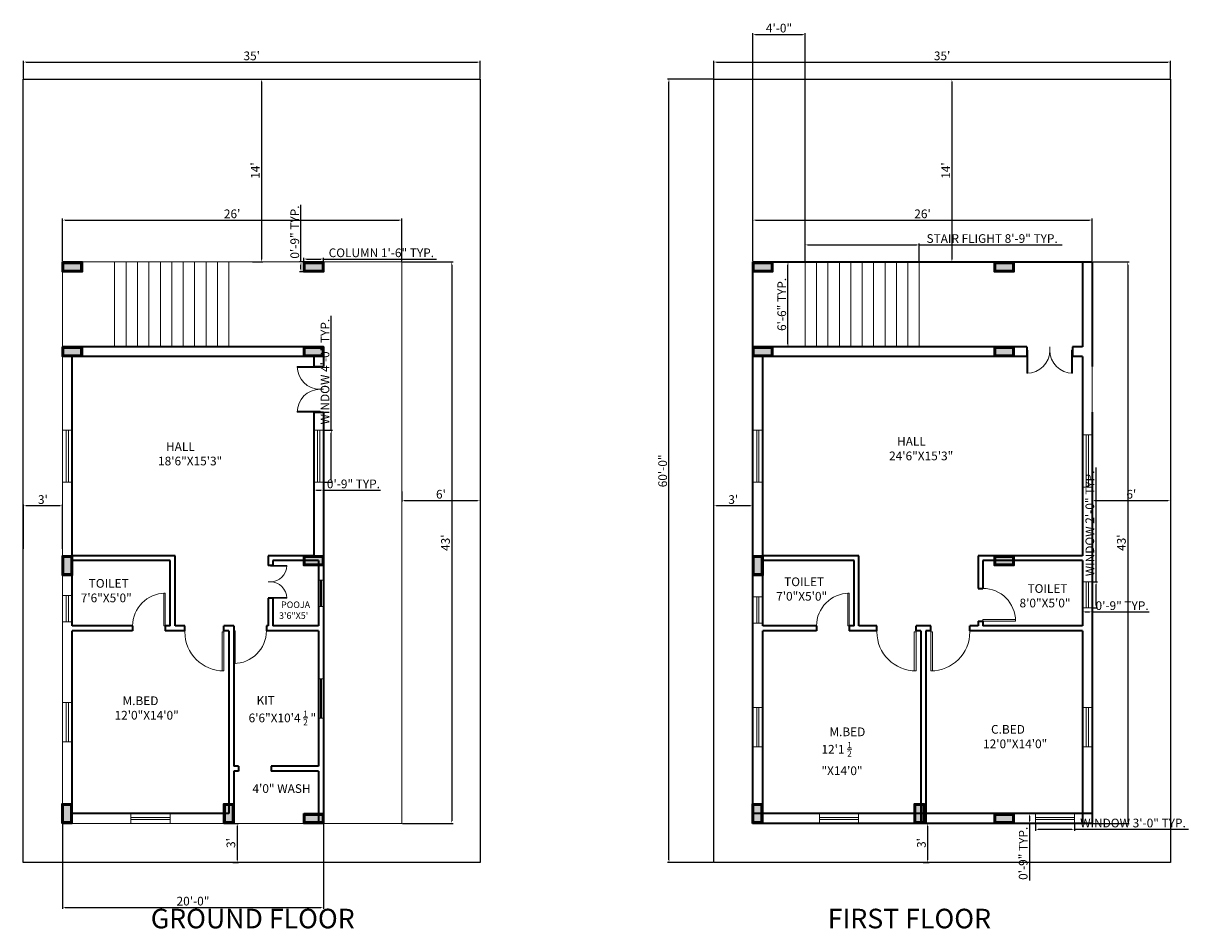
# Model space of a CAD drawing. Units: inches. Extents: x 538 to 2251, y 1112 to 1944.
# Tile 2 of 2: x 1179 to 2251, y 1112 to 1944. Entities that reach past the tile are written whole.
import ezdxf

# ---------------------------------------------------------------- set-up
doc = ezdxf.new("R2010")
doc.units = ezdxf.units.IN
for name, color, linetype, lineweight in [('A-AREA-IDEN', 7, 'Continuous', 18), ('A-FLOR-OTLN', 7, 'Continuous', 18), ('C-PROP', 7, 'Continuous', 25), ('COL', 6, 'Continuous', 35), ('DIMENSIONS', 6, 'Continuous', 18), ('DOORS', 2, 'Continuous', 18), ('STAIRS', 1, 'Continuous', 18), ('TEXT', 7, 'Continuous', 25), ('WALLS', 7, 'Continuous', 35), ('WINDOWS', 4, 'Continuous', 18)]:
    doc.layers.add(name, color=color, linetype=linetype, lineweight=lineweight)
doc.styles.get("Standard").update_dxf_attribs({"font": 'arial.ttf'})
doc.dimstyles.new('ISO-25', dxfattribs={"dimtxt": 8, "dimasz": 2.5, "dimexe": 1.25, "dimexo": 0.625, "dimtad": 1, "dimdec": 1, "dimlunit": 4, "dimtxsty": 'Standard', "dimcen": 2.5, "dimadec": 0, "dimazin": 0, "dimtfac": 1, "dimtdec": 1, "dimtmove": 0, "dimatfit": 3, "dimfxl": 1, "dimarcsym": 0})

# ---------------------------------------------------------------- blocks, each defined once
blk = doc.blocks.new('*D7')
at = {"layer": 'Defpoints', "color": 0, "transparency": 16777216}
for p in [(1599.2, 1908.3), (1179.2, 1892.6), (1599.2, 1892.6)]:
    blk.add_point(p, dxfattribs=at)
at = {"layer": 'DIMENSIONS', "color": 0, "lineweight": -2, "transparency": 16777216}
for p, q in [((1179.2, 1893.2), (1179.2, 1909.6)), ((1181.7, 1908.3), (1596.7, 1908.3)), ((1599.2, 1893.2), (1599.2, 1909.6))]:
    blk.add_line(p, q, dxfattribs=at)
at = {"layer": 'DIMENSIONS', "color": 0, "transparency": 16777216}
for points in [[(1181.7, 1908.7), (1181.7, 1907.9), (1179.2, 1908.3)], [(1596.7, 1908.7), (1596.7, 1907.9), (1599.2, 1908.3)]]:
    blk.add_solid(points, dxfattribs=at)
at = {"layer": 'DIMENSIONS', "color": 0, "transparency": 16777216, "insert": (1389.2, 1913), "char_height": 8, "attachment_point": 5}
blk.add_mtext("35'", dxfattribs=at)
blk = doc.blocks.new('*D8')
at = {"layer": 'Defpoints', "color": 0, "transparency": 16777216}
for p in [(1527.2, 1763.1), (1215.2, 1724.6), (1527.2, 1724.6)]:
    blk.add_point(p, dxfattribs=at)
at = {"layer": 'DIMENSIONS', "color": 0, "lineweight": -2, "transparency": 16777216}
for p, q in [((1215.2, 1725.2), (1215.2, 1764.4)), ((1217.7, 1763.1), (1524.7, 1763.1)), ((1527.2, 1725.2), (1527.2, 1764.4))]:
    blk.add_line(p, q, dxfattribs=at)
at = {"layer": 'DIMENSIONS', "color": 0, "transparency": 16777216}
for points in [[(1217.7, 1763.5), (1217.7, 1762.7), (1215.2, 1763.1)], [(1524.7, 1763.5), (1524.7, 1762.7), (1527.2, 1763.1)]]:
    blk.add_solid(points, dxfattribs=at)
at = {"layer": 'DIMENSIONS', "color": 0, "transparency": 16777216, "insert": (1371.2, 1767.8), "char_height": 8, "attachment_point": 5}
blk.add_mtext("26'", dxfattribs=at)
blk = doc.blocks.new('*D9')
at = {"layer": 'Defpoints', "color": 0, "transparency": 16777216}
for p in [(1389.2, 1892.6), (1389.2, 1724.6), (1398.1, 1724.6)]:
    blk.add_point(p, dxfattribs=at)
at = {"layer": 'DIMENSIONS', "color": 0, "lineweight": -2, "transparency": 16777216}
for p, q in [((1389.8, 1892.6), (1399.4, 1892.6)), ((1398.1, 1890.1), (1398.1, 1727.1)), ((1389.8, 1724.6), (1399.4, 1724.6))]:
    blk.add_line(p, q, dxfattribs=at)
at = {"layer": 'DIMENSIONS', "color": 0, "transparency": 16777216}
for points in [[(1397.7, 1890.1), (1398.6, 1890.1), (1398.1, 1892.6)], [(1397.7, 1727.1), (1398.6, 1727.1), (1398.1, 1724.6)]]:
    blk.add_solid(points, dxfattribs=at)
at = {"layer": 'DIMENSIONS', "color": 0, "transparency": 16777216, "insert": (1393.5, 1808.6), "char_height": 8, "attachment_point": 5, "rotation": 90}
blk.add_mtext("14'", dxfattribs=at)
blk = doc.blocks.new('*D10')
at = {"layer": 'Defpoints', "color": 0, "transparency": 16777216}
for p in [(1527.2, 1514.2), (1599.2, 1514.2), (1599.2, 1505.4)]:
    blk.add_point(p, dxfattribs=at)
at = {"layer": 'DIMENSIONS', "color": 0, "lineweight": -2, "transparency": 16777216}
for p, q in [((1527.2, 1513.6), (1527.2, 1504.2)), ((1599.2, 1513.6), (1599.2, 1504.2)), ((1529.7, 1505.4), (1596.7, 1505.4))]:
    blk.add_line(p, q, dxfattribs=at)
at = {"layer": 'DIMENSIONS', "color": 0, "transparency": 16777216}
for points in [[(1529.7, 1505.8), (1529.7, 1505), (1527.2, 1505.4)], [(1596.7, 1505.8), (1596.7, 1505), (1599.2, 1505.4)]]:
    blk.add_solid(points, dxfattribs=at)
at = {"layer": 'DIMENSIONS', "color": 0, "transparency": 16777216, "insert": (1563.2, 1510.1), "char_height": 8, "attachment_point": 5}
blk.add_mtext("6'", dxfattribs=at)
blk = doc.blocks.new('*D11')
at = {"layer": 'Defpoints', "color": 0, "transparency": 16777216}
for p in [(1371.2, 1208.6), (1371.2, 1172.6), (1375.9, 1172.6)]:
    blk.add_point(p, dxfattribs=at)
at = {"layer": 'DIMENSIONS', "color": 0, "lineweight": -2, "transparency": 16777216}
for p, q in [((1371.8, 1208.6), (1377.1, 1208.6)), ((1375.9, 1206.1), (1375.9, 1175.1)), ((1371.8, 1172.6), (1377.1, 1172.6))]:
    blk.add_line(p, q, dxfattribs=at)
at = {"layer": 'DIMENSIONS', "color": 0, "transparency": 16777216}
for points in [[(1375.4, 1206.1), (1376.3, 1206.1), (1375.9, 1208.6)], [(1375.4, 1175.1), (1376.3, 1175.1), (1375.9, 1172.6)]]:
    blk.add_solid(points, dxfattribs=at)
at = {"layer": 'DIMENSIONS', "color": 0, "transparency": 16777216, "insert": (1371.1, 1190.6), "char_height": 8, "attachment_point": 5, "rotation": 90}
blk.add_mtext("3'", dxfattribs=at)
blk = doc.blocks.new('*D12')
at = {"layer": 'Defpoints', "color": 0, "transparency": 16777216}
for p in [(1179.2, 1500.5), (1179.2, 1460.1), (1215.2, 1460.1)]:
    blk.add_point(p, dxfattribs=at)
at = {"layer": 'DIMENSIONS', "color": 0, "lineweight": -2, "transparency": 16777216}
for p, q in [((1179.2, 1460.8), (1179.2, 1501.7)), ((1212.7, 1500.5), (1181.7, 1500.5)), ((1215.2, 1460.8), (1215.2, 1501.7))]:
    blk.add_line(p, q, dxfattribs=at)
at = {"layer": 'DIMENSIONS', "color": 0, "transparency": 16777216}
for points in [[(1181.7, 1500.9), (1181.7, 1500.1), (1179.2, 1500.5)], [(1212.7, 1500.9), (1212.7, 1500.1), (1215.2, 1500.5)]]:
    blk.add_solid(points, dxfattribs=at)
at = {"layer": 'DIMENSIONS', "color": 0, "transparency": 16777216, "insert": (1197.2, 1505.2), "char_height": 8, "attachment_point": 5}
blk.add_mtext("3'", dxfattribs=at)
blk = doc.blocks.new('*D14')
at = {"layer": 'Defpoints', "color": 0, "transparency": 16777216}
for p in [(1527.2, 1724.6), (1527.2, 1208.6), (1573.1, 1208.6)]:
    blk.add_point(p, dxfattribs=at)
at = {"layer": 'DIMENSIONS', "color": 0, "lineweight": -2, "transparency": 16777216}
for p, q in [((1527.8, 1724.6), (1574.4, 1724.6)), ((1573.1, 1722.1), (1573.1, 1211.1)), ((1527.8, 1208.6), (1574.4, 1208.6))]:
    blk.add_line(p, q, dxfattribs=at)
at = {"layer": 'DIMENSIONS', "color": 0, "transparency": 16777216}
for points in [[(1572.7, 1722.1), (1573.5, 1722.1), (1573.1, 1724.6)], [(1572.7, 1211.1), (1573.5, 1211.1), (1573.1, 1208.6)]]:
    blk.add_solid(points, dxfattribs=at)
at = {"layer": 'DIMENSIONS', "color": 0, "transparency": 16777216, "insert": (1568.4, 1466.6), "char_height": 8, "attachment_point": 5, "rotation": 90}
blk.add_mtext("43'", dxfattribs=at)
blk = doc.blocks.new('*D15')
at = {"layer": 'Defpoints', "color": 0, "transparency": 16777216}
for p in [(2234, 1908.3), (1814, 1892.6), (2234, 1892.6)]:
    blk.add_point(p, dxfattribs=at)
at = {"layer": 'DIMENSIONS', "color": 0, "lineweight": -2, "transparency": 16777216}
for p, q in [((1814, 1893.2), (1814, 1909.6)), ((1816.5, 1908.3), (2231.5, 1908.3)), ((2234, 1893.2), (2234, 1909.6))]:
    blk.add_line(p, q, dxfattribs=at)
at = {"layer": 'DIMENSIONS', "color": 0, "transparency": 16777216}
for points in [[(1816.5, 1908.7), (1816.5, 1907.9), (1814, 1908.3)], [(2231.5, 1908.7), (2231.5, 1907.9), (2234, 1908.3)]]:
    blk.add_solid(points, dxfattribs=at)
at = {"layer": 'DIMENSIONS', "color": 0, "transparency": 16777216, "insert": (2024, 1913), "char_height": 8, "attachment_point": 5}
blk.add_mtext("35'", dxfattribs=at)
blk = doc.blocks.new('*D16')
at = {"layer": 'Defpoints', "color": 0, "transparency": 16777216}
for p in [(2162, 1763.1), (1850, 1724.6), (2162, 1724.6)]:
    blk.add_point(p, dxfattribs=at)
at = {"layer": 'DIMENSIONS', "color": 0, "lineweight": -2, "transparency": 16777216}
for p, q in [((1850, 1725.2), (1850, 1764.4)), ((1852.5, 1763.1), (2159.5, 1763.1)), ((2162, 1725.2), (2162, 1764.4))]:
    blk.add_line(p, q, dxfattribs=at)
at = {"layer": 'DIMENSIONS', "color": 0, "transparency": 16777216}
for points in [[(1852.5, 1763.5), (1852.5, 1762.7), (1850, 1763.1)], [(2159.5, 1763.5), (2159.5, 1762.7), (2162, 1763.1)]]:
    blk.add_solid(points, dxfattribs=at)
at = {"layer": 'DIMENSIONS', "color": 0, "transparency": 16777216, "insert": (2006, 1767.8), "char_height": 8, "attachment_point": 5}
blk.add_mtext("26'", dxfattribs=at)
blk = doc.blocks.new('*D17')
at = {"layer": 'Defpoints', "color": 0, "transparency": 16777216}
for p in [(2024, 1892.6), (2024, 1724.6), (2033, 1724.6)]:
    blk.add_point(p, dxfattribs=at)
at = {"layer": 'DIMENSIONS', "color": 0, "lineweight": -2, "transparency": 16777216}
for p, q in [((2024.7, 1892.6), (2034.2, 1892.6)), ((2033, 1890.1), (2033, 1727.1)), ((2024.7, 1724.6), (2034.2, 1724.6))]:
    blk.add_line(p, q, dxfattribs=at)
at = {"layer": 'DIMENSIONS', "color": 0, "transparency": 16777216}
for points in [[(2032.6, 1890.1), (2033.4, 1890.1), (2033, 1892.6)], [(2032.6, 1727.1), (2033.4, 1727.1), (2033, 1724.6)]]:
    blk.add_solid(points, dxfattribs=at)
at = {"layer": 'DIMENSIONS', "color": 0, "transparency": 16777216, "insert": (2028.4, 1808.6), "char_height": 8, "attachment_point": 5, "rotation": 90}
blk.add_mtext("14'", dxfattribs=at)
blk = doc.blocks.new('*D18')
at = {"layer": 'Defpoints', "color": 0, "transparency": 16777216}
for p in [(2162, 1514.2), (2234, 1514.2), (2234, 1505.4)]:
    blk.add_point(p, dxfattribs=at)
at = {"layer": 'DIMENSIONS', "color": 0, "lineweight": -2, "transparency": 16777216}
for p, q in [((2162, 1513.6), (2162, 1504.2)), ((2234, 1513.6), (2234, 1504.2)), ((2164.5, 1505.4), (2231.5, 1505.4))]:
    blk.add_line(p, q, dxfattribs=at)
at = {"layer": 'DIMENSIONS', "color": 0, "transparency": 16777216}
for points in [[(2164.5, 1505.8), (2164.5, 1505), (2162, 1505.4)], [(2231.5, 1505.8), (2231.5, 1505), (2234, 1505.4)]]:
    blk.add_solid(points, dxfattribs=at)
at = {"layer": 'DIMENSIONS', "color": 0, "transparency": 16777216, "insert": (2198, 1510.1), "char_height": 8, "attachment_point": 5}
blk.add_mtext("6'", dxfattribs=at)
blk = doc.blocks.new('*D19')
at = {"layer": 'Defpoints', "color": 0, "transparency": 16777216}
for p in [(2006, 1208.6), (2006, 1172.6), (2010.7, 1172.6)]:
    blk.add_point(p, dxfattribs=at)
at = {"layer": 'DIMENSIONS', "color": 0, "lineweight": -2, "transparency": 16777216}
for p, q in [((2006.7, 1208.6), (2012, 1208.6)), ((2010.7, 1206.1), (2010.7, 1175.1)), ((2006.7, 1172.6), (2012, 1172.6))]:
    blk.add_line(p, q, dxfattribs=at)
at = {"layer": 'DIMENSIONS', "color": 0, "transparency": 16777216}
for points in [[(2010.3, 1206.1), (2011.1, 1206.1), (2010.7, 1208.6)], [(2010.3, 1175.1), (2011.1, 1175.1), (2010.7, 1172.6)]]:
    blk.add_solid(points, dxfattribs=at)
at = {"layer": 'DIMENSIONS', "color": 0, "transparency": 16777216, "insert": (2006, 1190.6), "char_height": 8, "attachment_point": 5, "rotation": 90}
blk.add_mtext("3'", dxfattribs=at)
blk = doc.blocks.new('*D20')
at = {"layer": 'Defpoints', "color": 0, "transparency": 16777216}
for p in [(1814, 1500.5), (1814, 1460.1), (1850, 1460.1)]:
    blk.add_point(p, dxfattribs=at)
at = {"layer": 'DIMENSIONS', "color": 0, "lineweight": -2, "transparency": 16777216}
for p, q in [((1814, 1460.8), (1814, 1501.7)), ((1847.5, 1500.5), (1816.5, 1500.5)), ((1850, 1460.8), (1850, 1501.7))]:
    blk.add_line(p, q, dxfattribs=at)
at = {"layer": 'DIMENSIONS', "color": 0, "transparency": 16777216}
for points in [[(1816.5, 1500.9), (1816.5, 1500.1), (1814, 1500.5)], [(1847.5, 1500.9), (1847.5, 1500.1), (1850, 1500.5)]]:
    blk.add_solid(points, dxfattribs=at)
at = {"layer": 'DIMENSIONS', "color": 0, "transparency": 16777216, "insert": (1832, 1505.2), "char_height": 8, "attachment_point": 5}
blk.add_mtext("3'", dxfattribs=at)
blk = doc.blocks.new('*D21')
at = {"layer": 'Defpoints', "color": 0, "transparency": 16777216}
for p in [(2162, 1724.6), (2162, 1208.6), (2194.7, 1208.6)]:
    blk.add_point(p, dxfattribs=at)
at = {"layer": 'DIMENSIONS', "color": 0, "lineweight": -2, "transparency": 16777216}
for p, q in [((2162.7, 1724.6), (2195.9, 1724.6)), ((2194.7, 1722.1), (2194.7, 1211.1)), ((2162.7, 1208.6), (2195.9, 1208.6))]:
    blk.add_line(p, q, dxfattribs=at)
at = {"layer": 'DIMENSIONS', "color": 0, "transparency": 16777216}
for points in [[(2194.2, 1722.1), (2195.1, 1722.1), (2194.7, 1724.6)], [(2194.2, 1211.1), (2195.1, 1211.1), (2194.7, 1208.6)]]:
    blk.add_solid(points, dxfattribs=at)
at = {"layer": 'DIMENSIONS', "color": 0, "transparency": 16777216, "insert": (2189.9, 1466.6), "char_height": 8, "attachment_point": 5, "rotation": 90}
blk.add_mtext("43'", dxfattribs=at)
blk = doc.blocks.new('*U23')
for p, q in [((0, 0), (0, -6)), ((40, 0), (40, -6))]:
    blk.add_line(p, q)
blk.add_lwpolyline([(0, 0), (0, 40), (1.75, 40), (1.75, 0)], close=True)
blk.add_arc((0, 0), 40, 0, 90)
blk = doc.blocks.new('COL-18X9IN')
h = blk.add_hatch(color=256)
h.dxf.hatch_style = 1
h.paths.add_polyline_path([(8, 3.5), (-8, 3.5), (-8, -3.5), (8, -3.5)])
for points in [[(-9, 4.5), (9, 4.5), (9, -4.5), (-9, -4.5)], [(-8, 3.5), (8, 3.5), (8, -3.5), (-8, -3.5)]]:
    blk.add_lwpolyline(points, close=True)
blk = doc.blocks.new('STAIR-FLIGHT-78IN')
for p, q in [((0, 0), (0, 78)), ((10.5, 0), (10.5, 78)), ((21, 0), (21, 78)), ((31.5, 0), (31.5, 78)), ((42, 0), (42, 78)), ((52.5, 0), (52.5, 78)), ((63, 0), (63, 78)), ((73.5, 0), (73.5, 78)), ((84, 0), (84, 78)), ((94.5, 0), (94.5, 78)), ((105, 0), (105, 78))]:
    blk.add_line(p, q)
blk = doc.blocks.new('WIN-36X9IN')
for p, q in [((-1, 0), (-1, 36)), ((1, 0), (1, 36))]:
    blk.add_line(p, q)
blk.add_lwpolyline([(-4.5, 0), (-4.5, 36), (4.5, 36), (4.5, 0)], close=True)
blk = doc.blocks.new('WIN-48X9IN')
for p, q in [((-1, 0), (-1, 48)), ((1, 0), (1, 48))]:
    blk.add_line(p, q)
blk.add_lwpolyline([(-4.5, 0), (-4.5, 48), (4.5, 48), (4.5, 0)], close=True)
blk = doc.blocks.new('WIN-24X9IN')
for p, q in [((-1, 0), (-1, 24)), ((1, 0), (1, 24))]:
    blk.add_line(p, q)
blk.add_lwpolyline([(-4.5, 0), (-4.5, 24), (4.5, 24), (4.5, 0)], close=True)
blk = doc.blocks.new('*D29')
at = {"layer": 'Defpoints', "color": 0, "transparency": 16777216}
for p in [(1455.2, 1727.3), (1437.2, 1724.6), (1455.2, 1724.6)]:
    blk.add_point(p, dxfattribs=at)
at = {"layer": 'DIMENSIONS', "color": 0, "lineweight": -2, "transparency": 16777216}
for p, q in [((1437.2, 1725.2), (1437.2, 1728.5)), ((1439.7, 1727.3), (1452.7, 1727.3)), ((1455.2, 1725.2), (1455.2, 1728.5)), ((1455.2, 1727.3), (1559.1, 1727.3))]:
    blk.add_line(p, q, dxfattribs=at)
at = {"layer": 'DIMENSIONS', "color": 0, "transparency": 16777216}
for points in [[(1439.7, 1727.7), (1439.7, 1726.9), (1437.2, 1727.3)], [(1452.7, 1727.7), (1452.7, 1726.9), (1455.2, 1727.3)]]:
    blk.add_solid(points, dxfattribs=at)
at = {"layer": 'DIMENSIONS', "color": 0, "transparency": 16777216, "insert": (1508.4, 1732), "char_height": 8, "attachment_point": 5}
blk.add_mtext('COLUMN 1\'-6" TYP.', dxfattribs=at)
blk = doc.blocks.new('*D30')
at = {"layer": 'Defpoints', "color": 0, "transparency": 16777216}
for p in [(1434.5, 1724.6), (1437.2, 1724.6), (1437.2, 1715.6)]:
    blk.add_point(p, dxfattribs=at)
at = {"layer": 'DIMENSIONS', "color": 0, "lineweight": -2, "transparency": 16777216}
for p, q in [((1434.5, 1724.6), (1434.5, 1777.1)), ((1436.6, 1724.6), (1433.2, 1724.6)), ((1436.6, 1715.6), (1433.2, 1715.6)), ((1434.5, 1718.1), (1434.5, 1722.1))]:
    blk.add_line(p, q, dxfattribs=at)
at = {"layer": 'DIMENSIONS', "color": 0, "transparency": 16777216}
for points in [[(1434.1, 1722.1), (1434.9, 1722.1), (1434.5, 1724.6)], [(1434.1, 1718.1), (1434.9, 1718.1), (1434.5, 1715.6)]]:
    blk.add_solid(points, dxfattribs=at)
at = {"layer": 'DIMENSIONS', "color": 0, "transparency": 16777216, "insert": (1429.8, 1752.1), "char_height": 8, "attachment_point": 5, "rotation": 90}
blk.add_mtext('0\'-9" TYP.', dxfattribs=at)
blk = doc.blocks.new('*D31')
at = {"layer": 'Defpoints', "color": 0, "transparency": 16777216}
for p in [(2109.8, 1208.6), (2145.8, 1208.6), (2145.8, 1203.2)]:
    blk.add_point(p, dxfattribs=at)
at = {"layer": 'DIMENSIONS', "color": 0, "lineweight": -2, "transparency": 16777216}
for p, q in [((2109.8, 1208), (2109.8, 1201.9)), ((2112.3, 1203.2), (2143.3, 1203.2)), ((2145.8, 1208), (2145.8, 1201.9)), ((2145.8, 1203.2), (2250.7, 1203.2))]:
    blk.add_line(p, q, dxfattribs=at)
at = {"layer": 'DIMENSIONS', "color": 0, "transparency": 16777216}
for points in [[(2112.3, 1203.6), (2112.3, 1202.8), (2109.8, 1203.2)], [(2143.3, 1203.6), (2143.3, 1202.8), (2145.8, 1203.2)]]:
    blk.add_solid(points, dxfattribs=at)
at = {"layer": 'DIMENSIONS', "color": 0, "transparency": 16777216, "insert": (2199.5, 1207.9), "char_height": 8, "attachment_point": 5}
blk.add_mtext('WINDOW 3\'-0" TYP.', dxfattribs=at)
blk = doc.blocks.new('*D32')
at = {"layer": 'Defpoints', "color": 0, "transparency": 16777216}
for p in [(2109.8, 1217.6), (2104.4, 1208.6), (2109.8, 1208.6)]:
    blk.add_point(p, dxfattribs=at)
at = {"layer": 'DIMENSIONS', "color": 0, "lineweight": -2, "transparency": 16777216}
for p, q in [((2109.1, 1217.6), (2103.1, 1217.6)), ((2104.4, 1215.1), (2104.4, 1211.1)), ((2109.1, 1208.6), (2103.1, 1208.6)), ((2104.4, 1208.6), (2104.4, 1156.1))]:
    blk.add_line(p, q, dxfattribs=at)
at = {"layer": 'DIMENSIONS', "color": 0, "transparency": 16777216}
for points in [[(2103.9, 1215.1), (2104.8, 1215.1), (2104.4, 1217.6)], [(2103.9, 1211.1), (2104.8, 1211.1), (2104.4, 1208.6)]]:
    blk.add_solid(points, dxfattribs=at)
at = {"layer": 'DIMENSIONS', "color": 0, "transparency": 16777216, "insert": (2099.6, 1181.1), "char_height": 8, "attachment_point": 5, "rotation": 90}
blk.add_mtext('0\'-9" TYP.', dxfattribs=at)
blk = doc.blocks.new('*D33')
at = {"layer": 'Defpoints', "color": 0, "transparency": 16777216}
for p in [(1455.2, 1570.1), (1462.4, 1570.1), (1455.2, 1522.1)]:
    blk.add_point(p, dxfattribs=at)
at = {"layer": 'DIMENSIONS', "color": 0, "lineweight": -2, "transparency": 16777216}
for p, q in [((1462.4, 1570.1), (1462.4, 1675.1)), ((1455.8, 1570.1), (1463.6, 1570.1)), ((1462.4, 1524.6), (1462.4, 1567.6)), ((1455.8, 1522.1), (1463.6, 1522.1))]:
    blk.add_line(p, q, dxfattribs=at)
at = {"layer": 'DIMENSIONS', "color": 0, "transparency": 16777216}
for points in [[(1462, 1567.6), (1462.8, 1567.6), (1462.4, 1570.1)], [(1462, 1524.6), (1462.8, 1524.6), (1462.4, 1522.1)]]:
    blk.add_solid(points, dxfattribs=at)
at = {"layer": 'DIMENSIONS', "color": 0, "transparency": 16777216, "insert": (1457.6, 1623.8), "char_height": 8, "attachment_point": 5, "rotation": 90}
blk.add_mtext('WINDOW 4\'-0" TYP.', dxfattribs=at)
blk = doc.blocks.new('*D34')
at = {"layer": 'Defpoints', "color": 0, "transparency": 16777216}
for p in [(1446.2, 1522.1), (1455.2, 1522.1), (1455.2, 1514.9)]:
    blk.add_point(p, dxfattribs=at)
at = {"layer": 'DIMENSIONS', "color": 0, "lineweight": -2, "transparency": 16777216}
for p, q in [((1446.2, 1521.5), (1446.2, 1513.6)), ((1448.7, 1514.9), (1452.7, 1514.9)), ((1455.2, 1521.5), (1455.2, 1513.6)), ((1455.2, 1514.9), (1507.7, 1514.9))]:
    blk.add_line(p, q, dxfattribs=at)
at = {"layer": 'DIMENSIONS', "color": 0, "transparency": 16777216}
for points in [[(1448.7, 1515.3), (1448.7, 1514.5), (1446.2, 1514.9)], [(1452.7, 1515.3), (1452.7, 1514.5), (1455.2, 1514.9)]]:
    blk.add_solid(points, dxfattribs=at)
at = {"layer": 'DIMENSIONS', "color": 0, "transparency": 16777216, "insert": (1482.7, 1519.6), "char_height": 8, "attachment_point": 5}
blk.add_mtext('0\'-9" TYP.', dxfattribs=at)
blk = doc.blocks.new('*D35')
at = {"layer": 'Defpoints', "color": 0, "transparency": 16777216}
for p in [(2162, 1430.6), (2165.6, 1430.6), (2162, 1406.6)]:
    blk.add_point(p, dxfattribs=at)
at = {"layer": 'DIMENSIONS', "color": 0, "lineweight": -2, "transparency": 16777216}
for p, q in [((2165.6, 1430.6), (2165.6, 1535.6)), ((2162.7, 1430.6), (2166.9, 1430.6)), ((2165.6, 1409.1), (2165.6, 1428.1)), ((2162.7, 1406.6), (2166.9, 1406.6))]:
    blk.add_line(p, q, dxfattribs=at)
at = {"layer": 'DIMENSIONS', "color": 0, "transparency": 16777216}
for points in [[(2165.2, 1428.1), (2166.1, 1428.1), (2165.6, 1430.6)], [(2165.2, 1409.1), (2166.1, 1409.1), (2165.6, 1406.6)]]:
    blk.add_solid(points, dxfattribs=at)
at = {"layer": 'DIMENSIONS', "color": 0, "transparency": 16777216, "insert": (2160.9, 1484.3), "char_height": 8, "attachment_point": 5, "rotation": 90}
blk.add_mtext('WINDOW 2\'-0" TYP.', dxfattribs=at)
blk = doc.blocks.new('*D36')
at = {"layer": 'Defpoints', "color": 0, "transparency": 16777216}
for p in [(2153, 1406.6), (2162, 1406.6), (2162, 1403)]:
    blk.add_point(p, dxfattribs=at)
at = {"layer": 'DIMENSIONS', "color": 0, "lineweight": -2, "transparency": 16777216}
for p, q in [((2153, 1406), (2153, 1401.7)), ((2162, 1406), (2162, 1401.7)), ((2155.5, 1403), (2159.5, 1403)), ((2162, 1403), (2214.5, 1403))]:
    blk.add_line(p, q, dxfattribs=at)
at = {"layer": 'DIMENSIONS', "color": 0, "transparency": 16777216}
for points in [[(2155.5, 1403.4), (2155.5, 1402.6), (2153, 1403)], [(2159.5, 1403.4), (2159.5, 1402.6), (2162, 1403)]]:
    blk.add_solid(points, dxfattribs=at)
at = {"layer": 'DIMENSIONS', "color": 0, "transparency": 16777216, "insert": (2189.5, 1407.7), "char_height": 8, "attachment_point": 5}
blk.add_mtext('0\'-9" TYP.', dxfattribs=at)
blk = doc.blocks.new('*D37')
at = {"layer": 'Defpoints', "color": 0, "transparency": 16777216}
for p in [(2003, 1740.3), (1898, 1724.6), (2003, 1724.6)]:
    blk.add_point(p, dxfattribs=at)
at = {"layer": 'DIMENSIONS', "color": 0, "lineweight": -2, "transparency": 16777216}
for p, q in [((1898, 1725.2), (1898, 1741.6)), ((1900.5, 1740.3), (2000.5, 1740.3)), ((2003, 1725.2), (2003, 1741.6)), ((2003, 1740.3), (2134.4, 1740.3))]:
    blk.add_line(p, q, dxfattribs=at)
at = {"layer": 'DIMENSIONS', "color": 0, "transparency": 16777216}
for points in [[(1900.5, 1740.7), (1900.5, 1739.9), (1898, 1740.3)], [(2000.5, 1740.7), (2000.5, 1739.9), (2003, 1740.3)]]:
    blk.add_solid(points, dxfattribs=at)
at = {"layer": 'DIMENSIONS', "color": 0, "transparency": 16777216, "insert": (2070, 1745.1), "char_height": 8, "attachment_point": 5}
blk.add_mtext('STAIR FLIGHT 8\'-9" TYP.', dxfattribs=at)
blk = doc.blocks.new('*D38')
at = {"layer": 'Defpoints', "color": 0, "transparency": 16777216}
for p in [(1882.3, 1724.6), (1898, 1724.6), (1898, 1646.6)]:
    blk.add_point(p, dxfattribs=at)
at = {"layer": 'DIMENSIONS', "color": 0, "lineweight": -2, "transparency": 16777216}
for p, q in [((1897.4, 1724.6), (1881, 1724.6)), ((1882.3, 1649.1), (1882.3, 1722.1)), ((1897.4, 1646.6), (1881, 1646.6))]:
    blk.add_line(p, q, dxfattribs=at)
at = {"layer": 'DIMENSIONS', "color": 0, "transparency": 16777216}
for points in [[(1881.9, 1722.1), (1882.7, 1722.1), (1882.3, 1724.6)], [(1881.9, 1649.1), (1882.7, 1649.1), (1882.3, 1646.6)]]:
    blk.add_solid(points, dxfattribs=at)
at = {"layer": 'DIMENSIONS', "color": 0, "transparency": 16777216, "insert": (1877.6, 1685.6), "char_height": 8, "attachment_point": 5, "rotation": 90}
blk.add_mtext('6\'-6" TYP.', dxfattribs=at)
blk = doc.blocks.new('*D41')
at = {"layer": 'Defpoints', "color": 0, "transparency": 16777216}
for p in [(1772.8, 1892.6), (1814, 1892.6), (1814, 1172.6)]:
    blk.add_point(p, dxfattribs=at)
at = {"layer": 'DIMENSIONS', "color": 0, "lineweight": -2, "transparency": 16777216}
for p, q in [((1813.4, 1892.6), (1771.6, 1892.6)), ((1772.8, 1175.1), (1772.8, 1890.1)), ((1813.4, 1172.6), (1771.6, 1172.6))]:
    blk.add_line(p, q, dxfattribs=at)
at = {"layer": 'DIMENSIONS', "color": 0, "transparency": 16777216}
for points in [[(1772.4, 1890.1), (1773.3, 1890.1), (1772.8, 1892.6)], [(1772.4, 1175.1), (1773.3, 1175.1), (1772.8, 1172.6)]]:
    blk.add_solid(points, dxfattribs=at)
at = {"layer": 'DIMENSIONS', "color": 0, "transparency": 16777216, "insert": (1768.1, 1532.6), "char_height": 8, "attachment_point": 5, "rotation": 90}
blk.add_mtext('60\'-0"', dxfattribs=at)
blk = doc.blocks.new('*D42')
at = {"layer": 'Defpoints', "color": 0, "transparency": 16777216}
for p in [(1215.2, 1208.6), (1455.2, 1208.6), (1455.2, 1131.4)]:
    blk.add_point(p, dxfattribs=at)
at = {"layer": 'DIMENSIONS', "color": 0, "lineweight": -2, "transparency": 16777216}
for p, q in [((1215.2, 1208), (1215.2, 1130.1)), ((1455.2, 1208), (1455.2, 1130.1)), ((1217.7, 1131.4), (1452.7, 1131.4))]:
    blk.add_line(p, q, dxfattribs=at)
at = {"layer": 'DIMENSIONS', "color": 0, "transparency": 16777216}
for points in [[(1217.7, 1131.8), (1217.7, 1131), (1215.2, 1131.4)], [(1452.7, 1131.8), (1452.7, 1131), (1455.2, 1131.4)]]:
    blk.add_solid(points, dxfattribs=at)
at = {"layer": 'DIMENSIONS', "color": 0, "transparency": 16777216, "insert": (1335.2, 1136.1), "char_height": 8, "attachment_point": 5}
blk.add_mtext('20\'-0"', dxfattribs=at)
blk = doc.blocks.new('*D43')
at = {"layer": 'Defpoints', "color": 0, "transparency": 16777216}
for p in [(1898, 1933.8), (1850, 1724.6), (1898, 1724.6)]:
    blk.add_point(p, dxfattribs=at)
at = {"layer": 'DIMENSIONS', "color": 0, "lineweight": -2, "transparency": 16777216}
for p, q in [((1850, 1725.2), (1850, 1935)), ((1852.5, 1933.8), (1895.5, 1933.8)), ((1898, 1725.2), (1898, 1935))]:
    blk.add_line(p, q, dxfattribs=at)
at = {"layer": 'DIMENSIONS', "color": 0, "transparency": 16777216}
for points in [[(1852.5, 1934.2), (1852.5, 1933.4), (1850, 1933.8)], [(1895.5, 1934.2), (1895.5, 1933.4), (1898, 1933.8)]]:
    blk.add_solid(points, dxfattribs=at)
at = {"layer": 'DIMENSIONS', "color": 0, "transparency": 16777216, "insert": (1874, 1938.5), "char_height": 8, "attachment_point": 5}
blk.add_mtext('4\'-0"', dxfattribs=at)

msp = doc.modelspace()

# ---------------------------------------------------------------- linework, layer by layer
at = {"layer": 'A-FLOR-OTLN'}
for p, q in [((1215.18, 1724.58), (1527.18, 1724.58)), ((1215.18, 1208.58), (1215.18, 1724.58)), ((1527.18, 1724.58), (1527.18, 1208.58)), ((1850.03, 1724.58), (2162.03, 1724.58)), ((1850.03, 1208.58), (1850.03, 1724.58)), ((2162.03, 1724.58), (2162.03, 1628.58)), ((2162.03, 1628.58), (2162.03, 1208.58)), ((1527.18, 1208.58), (1215.18, 1208.58)), ((2162.03, 1208.58), (1850.03, 1208.58))]:
    msp.add_line(p, q, dxfattribs=at)
at = {"layer": 'C-PROP'}
for p, q in [((1179.18, 1892.58), (1599.18, 1892.58)), ((1179.18, 1172.58), (1179.18, 1892.58)), ((1599.18, 1892.58), (1599.18, 1172.58)), ((1814.03, 1892.58), (2234.03, 1892.58)), ((1814.03, 1172.58), (1814.03, 1892.58)), ((2234.03, 1892.58), (2234.03, 1172.58)), ((1599.18, 1172.58), (1179.18, 1172.58)), ((2234.03, 1172.58), (1814.03, 1172.58))]:
    msp.add_line(p, q, dxfattribs=at)
at = {"layer": 'WALLS'}
for p, q in [((1850.03, 1724.58), (2162.03, 1724.58)), ((1850.03, 1208.58), (1850.03, 1724.58)), ((2153.03, 1724.58), (2153.03, 1646.58)), ((2162.03, 1724.58), (2162.03, 1628.58)), ((1455.18, 1646.58), (1215.18, 1646.58)), ((1455.18, 1646.58), (1455.18, 1628.58)), ((2102.03, 1646.58), (1850.03, 1646.58)), ((2102.03, 1646.58), (2102.03, 1637.58)), ((2153.03, 1646.58), (2144.03, 1646.58)), ((2144.03, 1646.58), (2144.03, 1637.58)), ((1446.18, 1637.58), (1224.18, 1637.58)), ((1224.18, 1454.58), (1224.18, 1637.58)), ((1446.18, 1637.58), (1446.18, 1628.58)), ((1859.03, 1454.58), (1859.03, 1637.58)), ((2102.03, 1637.58), (1859.03, 1637.58)), ((2153.03, 1637.58), (2144.03, 1637.58)), ((2153.03, 1637.58), (2153.03, 1628.58)), ((1446.18, 1628.58), (1455.18, 1628.58)), ((2153.03, 1628.58), (2153.03, 1454.58)), ((1446.18, 1586.58), (1455.18, 1586.58)), ((1446.18, 1586.58), (1446.18, 1454.58)), ((1455.18, 1586.58), (1455.18, 1208.58)), ((2162.03, 1586.58), (2162.03, 1208.58)), ((1318.68, 1454.58), (1224.18, 1454.58)), ((1314.18, 1450.08), (1224.18, 1450.08)), ((1224.18, 1390.08), (1224.18, 1450.08)), ((1314.18, 1390.08), (1314.18, 1450.08)), ((1318.68, 1390.08), (1318.68, 1454.58)), ((1446.18, 1454.58), (1404.18, 1454.58)), ((1404.18, 1454.58), (1404.18, 1445.58)), ((1450.68, 1450.08), (1408.68, 1450.08)), ((1408.68, 1450.08), (1408.68, 1445.58)), ((1450.68, 1450.08), (1450.68, 1390.08)), ((1947.53, 1454.58), (1859.03, 1454.58)), ((1943.03, 1450.08), (1859.03, 1450.08)), ((1859.03, 1390.08), (1859.03, 1450.08)), ((1943.03, 1390.08), (1943.03, 1450.08)), ((1947.53, 1390.08), (1947.53, 1454.58)), ((2057.03, 1454.58), (2057.03, 1424.58)), ((2153.03, 1454.58), (2057.03, 1454.58)), ((2061.53, 1450.08), (2061.53, 1424.58)), ((2153.03, 1450.08), (2061.53, 1450.08)), ((2153.03, 1450.08), (2153.03, 1390.08)), ((1408.68, 1445.58), (1404.18, 1445.58)), ((1408.68, 1415.58), (1404.18, 1415.58)), ((1404.18, 1415.58), (1404.18, 1390.08)), ((1408.68, 1415.58), (1408.68, 1390.08)), ((2057.03, 1424.58), (2061.53, 1424.58)), ((2057.03, 1394.58), (2061.53, 1394.58)), ((2057.03, 1394.58), (2057.03, 1390.08)), ((2061.53, 1394.58), (2061.53, 1390.08)), ((1279.68, 1390.08), (1224.18, 1390.08)), ((1224.18, 1217.58), (1224.18, 1385.58)), ((1279.68, 1385.58), (1224.18, 1385.58)), ((1279.68, 1390.08), (1279.68, 1385.58)), ((1314.18, 1390.08), (1309.68, 1390.08)), ((1309.68, 1390.08), (1309.68, 1385.58)), ((1327.68, 1385.58), (1309.68, 1385.58)), ((1327.68, 1390.08), (1318.68, 1390.08)), ((1327.68, 1385.58), (1327.68, 1390.08)), ((1363.68, 1385.58), (1363.68, 1390.08)), ((1372.68, 1390.08), (1363.68, 1390.08)), ((1368.18, 1385.58), (1363.68, 1385.58)), ((1368.18, 1385.58), (1368.18, 1217.58)), ((1372.68, 1390.08), (1372.68, 1261.08)), ((1404.18, 1390.08), (1402.68, 1390.08)), ((1402.68, 1390.08), (1402.68, 1385.58)), ((1450.68, 1385.58), (1402.68, 1385.58)), ((1450.68, 1390.08), (1408.68, 1390.08)), ((1450.68, 1385.58), (1450.68, 1261.08)), ((1908.53, 1390.08), (1859.03, 1390.08)), ((1859.03, 1208.58), (1859.03, 1385.58)), ((1908.53, 1385.58), (1859.03, 1385.58)), ((1908.53, 1390.08), (1908.53, 1385.58)), ((1943.03, 1390.08), (1938.53, 1390.08)), ((1938.53, 1390.08), (1938.53, 1385.58)), ((1964.03, 1385.58), (1938.53, 1385.58)), ((1964.03, 1390.08), (1947.53, 1390.08)), ((1964.03, 1385.58), (1964.03, 1390.08)), ((2013.53, 1390.08), (2000.03, 1390.08)), ((2000.03, 1385.58), (2000.03, 1390.08)), ((2004.53, 1385.58), (2000.03, 1385.58)), ((2004.53, 1385.58), (2004.53, 1208.58)), ((2009.03, 1385.58), (2009.03, 1208.58)), ((2013.53, 1385.58), (2009.03, 1385.58)), ((2013.53, 1385.58), (2013.53, 1390.08)), ((2057.03, 1390.08), (2049.53, 1390.08)), ((2049.53, 1385.58), (2049.53, 1390.08)), ((2153.03, 1385.58), (2049.53, 1385.58)), ((2153.03, 1390.08), (2061.53, 1390.08)), ((2153.03, 1385.58), (2153.03, 1208.58)), ((1377.18, 1261.08), (1372.68, 1261.08)), ((1372.68, 1256.58), (1372.68, 1208.58)), ((1377.18, 1256.58), (1372.68, 1256.58)), ((1377.18, 1261.08), (1377.18, 1256.58)), ((1450.68, 1261.08), (1407.18, 1261.08)), ((1407.18, 1261.08), (1407.18, 1256.58)), ((1450.68, 1256.58), (1407.18, 1256.58)), ((1450.68, 1256.58), (1450.68, 1208.58)), ((1368.18, 1217.58), (1224.18, 1217.58)), ((2162.03, 1217.58), (1850.03, 1217.58)), ((2162.03, 1208.58), (1850.03, 1208.58))]:
    msp.add_line(p, q, dxfattribs=at)
at = {"layer": 'WINDOWS'}
for p, q in [((1452.43, 1432.08), (1452.43, 1408.08)), ((1453.43, 1432.08), (1453.43, 1408.08)), ((1450.68, 1305.33), (1450.68, 1341.33)), ((1450.68, 1341.33), (1455.18, 1341.33)), ((1452.43, 1341.33), (1452.43, 1305.33)), ((1453.43, 1341.33), (1453.43, 1305.33)), ((1455.18, 1341.33), (1455.18, 1305.33)), ((1455.18, 1305.33), (1450.68, 1305.33))]:
    msp.add_line(p, q, dxfattribs=at)
msp.add_lwpolyline([(1450.68, 1432.08), (1455.18, 1432.08), (1455.18, 1408.08), (1450.68, 1408.08)], close=True, dxfattribs=at)

# ---------------------------------------------------------------- block references
at = {"layer": 'COL'}
for p in [(1224.18, 1720.08), (1446.18, 1720.08), (1859.03, 1720.08), (2081.03, 1720.08), (1224.18, 1642.08), (1446.18, 1642.08), (1859.03, 1642.08), (2081.03, 1642.08), (1446.18, 1450.08), (2081.03, 1450.08), (1446.18, 1213.08), (2081.03, 1213.08)]:
    msp.add_blockref('COL-18X9IN', p, dxfattribs=at)
for p, rotation in [((1219.68, 1445.58), 90.0000000000057), ((1854.53, 1445.58), 90.00000000000777), ((1219.33, 1217.58), 90.00000000000786), ((1368.18, 1217.58), 90.0000000000057), ((1854.19, 1217.58), 90.00000000000684), ((2003.03, 1217.58), 90.0000000000036)]:
    msp.add_blockref('COL-18X9IN', p, dxfattribs=dict(at, rotation=rotation))
at = {"layer": 'DOORS'}
for p, xscale, yscale, zscale, rotation in [((2102.03, 1643.43), -0.525, 0.525, 0.525, 180), ((2144.03, 1643.43), 0.525, 0.525, 0.525, 180), ((1452.03, 1628.58), -0.525, 0.525, 0.525, 90), ((1452.03, 1586.58), 0.525, 0.525, 0.525, 90), ((1406.43, 1445.58), 0.375, 0.375, 0.375, 270), ((1406.43, 1415.58), -0.375, 0.375, 0.375, 270), ((2061.53, 1394.58), -0.75, 0.75, 0.75, 270), ((1363.68, 1384.68), 0.9, 0.9, 0.9, 180), ((1372.68, 1385.58), -0.75, 0.75, 0.75, 180), ((2000.03, 1384.68), 0.9, 0.9, 0.9, 180), ((2013.53, 1384.68), -0.9, 0.9, 0.9, 180)]:
    msp.add_blockref('*U23', p, dxfattribs=dict(at, xscale=xscale, yscale=yscale, zscale=zscale, rotation=rotation))
at = {"layer": 'DOORS', "xscale": -0.75, "yscale": 0.75, "zscale": 0.75}
for p in [(1309.68, 1390.08), (1938.53, 1390.08)]:
    msp.add_blockref('*U23', p, dxfattribs=at)
at = {"layer": 'STAIRS'}
for p in [(1263.18, 1646.58), (1898.03, 1646.58)]:
    msp.add_blockref('STAIR-FLIGHT-78IN', p, dxfattribs=at)
at = {"layer": 'WINDOWS'}
for name, p in [('WIN-48X9IN', (1219.68, 1522.08)), ('WIN-48X9IN', (1450.68, 1522.08)), ('WIN-48X9IN', (1854.53, 1522.08)), ('WIN-48X9IN', (2157.53, 1517.58)), ('WIN-24X9IN', (2157.53, 1406.58)), ('WIN-24X9IN', (1219.68, 1393.97)), ('WIN-24X9IN', (1854.53, 1392.71)), ('WIN-36X9IN', (1219.68, 1283.58)), ('WIN-36X9IN', (1854.53, 1279.08)), ('WIN-36X9IN', (2157.53, 1279.08))]:
    msp.add_blockref(name, p, dxfattribs=at)
for p, rotation in [((1278.18, 1213.08), 269.9999999999994), ((1911.28, 1213.08), 269.9999999999997), ((2109.76, 1213.08), 270)]:
    msp.add_blockref('WIN-36X9IN', p, dxfattribs=dict(at, rotation=rotation))

# ---------------------------------------------------------------- texts
at = {"layer": 'A-AREA-IDEN', "attachment_point": 1}
for s, insert, char_height in [('   HALL\\P18\'6"X15\'3"', (1303.08, 1558.98), 8), ('   HALL\\P24\'6"X15\'3"', (1975.26, 1563.68), 8), ('   TOILET\\P7\'6"X5\'0"', (1231.99, 1433.2), 8), ('   TOILET\\P7\'0"X5\'0"', (1871.42, 1434.66), 8), ('   TOILET\\P8\'0"X5\'0"', (2095.19, 1428.47), 8), ('\\A1; POOJA\\P3\'6"X5\'', (1414.35, 1412.57), 6), ('   M.BED\\P12\'0"X14\'0"', (1263.09, 1325.33), 8), ('\\A1;   KIT\\P6\'6"X10\'4 {\\H0.7x;\\S1/2;} "', (1386.32, 1325.59), 8), ('\\A1;   M.BED\\P12\'1 {\\H0.7x;\\S1/2;} "X14\'0"', (1913.07, 1296.76), 8), ('   C.BED\\P12\'0"X14\'0"', (2061.68, 1299.04), 8), ('  4\'0" WASH', (1384.98, 1244.58), 8)]:
    msp.add_mtext_dynamic_manual_height_columns(s, width=67.8304, gutter_width=12.5, heights=[0], dxfattribs=dict(at, insert=insert, char_height=char_height))
at = {"layer": 'TEXT', "char_height": 18, "attachment_point": 1}
for s, insert in [('GROUND FLOOR', (1296.38, 1130.15)), ('FIRST FLOOR', (1918.88, 1130.15))]:
    msp.add_mtext_dynamic_manual_height_columns(s, width=205.0176, gutter_width=12.5, heights=[0], dxfattribs=dict(at, insert=insert))

# ---------------------------------------------------------------- dimensions: what is measured, and where the dimension line sits
at = {"layer": 'DIMENSIONS'}
for base, p1, p2, override, picture, middle in [((1898.03, 1933.78), (1850.03, 1724.58), (1898.03, 1724.58), {"dimdec": 1, "dimlfac": 1, "dimrnd": 0, "dimzin": 1, "dimdsep": 46, "dimlunit": 4, "dimfrac": 2}, '*D43', (1874.03, 1938.49)), ((1599.18, 1908.31), (1179.18, 1892.58), (1599.18, 1892.58), {"dimclrd": 0, "dimclre": 0, "dimclrt": 0}, '*D7', (1389.18, 1913.02)), ((2234.03, 1908.31), (1814.03, 1892.58), (2234.03, 1892.58), {"dimclrd": 0, "dimclre": 0, "dimclrt": 0}, '*D15', (2024.03, 1913.02)), ((1527.18, 1763.11), (1215.18, 1724.58), (1527.18, 1724.58), {"dimclrd": 0, "dimclre": 0, "dimclrt": 0}, '*D8', (1371.18, 1767.82)), ((2162.03, 1763.11), (1850.03, 1724.58), (2162.03, 1724.58), {"dimclrd": 0, "dimclre": 0, "dimclrt": 0}, '*D16', (2006.03, 1767.82)), ((1599.18, 1505.41), (1527.18, 1514.21), (1599.18, 1514.21), {"dimclrd": 0, "dimclre": 0, "dimclrt": 0}, '*D10', (1563.18, 1510.11)), ((2234.03, 1505.41), (2162.03, 1514.21), (2234.03, 1514.21), {"dimclrd": 0, "dimclre": 0, "dimclrt": 0}, '*D18', (2198.03, 1510.11)), ((1179.18, 1500.48), (1215.18, 1460.13), (1179.18, 1460.13), {"dimclrd": 0, "dimclre": 0, "dimclrt": 0}, '*D12', (1197.18, 1505.19)), ((1814.03, 1500.48), (1850.03, 1460.13), (1814.03, 1460.13), {"dimclrd": 0, "dimclre": 0, "dimclrt": 0}, '*D20', (1832.03, 1505.19)), ((1455.18, 1131.38), (1215.18, 1208.58), (1455.18, 1208.58), {"dimdec": 1, "dimlfac": 1, "dimrnd": 0, "dimzin": 1, "dimdsep": 46, "dimlunit": 4, "dimfrac": 2}, '*D42', (1335.18, 1136.09))]:
    dim = msp.add_linear_dim(base=base, p1=p1, p2=p2, dimstyle='ISO-25', override=override, dxfattribs=at)
    dim.commit()
    dim.dimension.update_dxf_attribs({"geometry": picture, "text_midpoint": middle})
for base, p1, p2, override, picture, middle in [((1398.13, 1724.58), (1389.18, 1892.58), (1389.18, 1724.58), {"dimclrd": 0, "dimclre": 0, "dimclrt": 0}, '*D9', (1393.49, 1808.58)), ((1772.83, 1892.58), (1814.03, 1172.58), (1814.03, 1892.58), {"dimdec": 1, "dimlfac": 1, "dimrnd": 0, "dimzin": 1, "dimdsep": 46, "dimlunit": 4, "dimfrac": 2}, '*D41', (1768.12, 1532.58)), ((2032.99, 1724.58), (2024.03, 1892.58), (2024.03, 1724.58), {"dimclrd": 0, "dimclre": 0, "dimclrt": 0}, '*D17', (2028.35, 1808.58)), ((1573.13, 1208.58), (1527.18, 1724.58), (1527.18, 1208.58), {"dimclrd": 0, "dimclre": 0, "dimclrt": 0}, '*D14', (1568.41, 1466.58)), ((2194.66, 1208.58), (2162.03, 1724.58), (2162.03, 1208.58), {"dimclrd": 0, "dimclre": 0, "dimclrt": 0}, '*D21', (2189.95, 1466.58)), ((1375.85, 1172.58), (1371.18, 1208.58), (1371.18, 1172.58), {"dimclrd": 0, "dimclre": 0, "dimclrt": 0}, '*D11', (1371.14, 1190.58)), ((2010.71, 1172.58), (2006.03, 1208.58), (2006.03, 1172.58), {"dimclrd": 0, "dimclre": 0, "dimclrt": 0}, '*D19', (2006, 1190.58))]:
    dim = msp.add_linear_dim(base=base, p1=p1, p2=p2, angle=90, dimstyle='ISO-25', override=override, dxfattribs=at)
    dim.commit()
    dim.dimension.update_dxf_attribs({"geometry": picture, "text_midpoint": middle})
for base, p1, p2, angle, text, picture, middle in [((1434.48, 1724.58), (1437.18, 1715.58), (1437.18, 1724.58), 90, '<> TYP.', '*D30', (1429.77, 1752.09)), ((1882.28, 1724.58), (1898.03, 1646.58), (1898.03, 1724.58), 90, '<> TYP.', '*D38', (1877.57, 1685.58)), ((1462.38, 1570.08), (1455.18, 1522.08), (1455.18, 1570.08), 90, 'WINDOW <> TYP.', '*D33', (1457.61, 1623.82)), ((2165.63, 1430.58), (2162.03, 1406.58), (2162.03, 1430.58), 90, 'WINDOW <> TYP.', '*D35', (2160.87, 1484.32)), ((2104.36, 1208.58), (2109.76, 1217.58), (2109.76, 1208.58), 270, '<> TYP.', '*D32', (2099.65, 1181.07))]:
    dim = msp.add_linear_dim(base=base, p1=p1, p2=p2, angle=angle, text=text, dimstyle='ISO-25', override={"dimdec": 1, "dimlfac": 1, "dimrnd": 0, "dimzin": 1, "dimdsep": 46, "dimlunit": 4, "dimfrac": 2}, dxfattribs=at)
    dim.commit()
    dim.dimension.update_dxf_attribs({"geometry": picture, "text_midpoint": middle})
for base, p1, p2, text, picture, middle in [((2003.03, 1740.33), (1898.03, 1724.58), (2003.03, 1724.58), 'STAIR FLIGHT <> TYP.', '*D37', (2069.95, 1745.09)), ((1455.18, 1727.28), (1437.18, 1724.58), (1455.18, 1724.58), 'COLUMN <> TYP.', '*D29', (1508.4, 1732.04)), ((1455.18, 1514.88), (1446.18, 1522.08), (1455.18, 1522.08), '<> TYP.', '*D34', (1482.68, 1519.59)), ((2162.03, 1402.98), (2153.03, 1406.58), (2162.03, 1406.58), '<> TYP.', '*D36', (2189.54, 1407.69)), ((2145.76, 1203.18), (2109.76, 1208.58), (2145.76, 1208.58), 'WINDOW <> TYP.', '*D31', (2199.5, 1207.95))]:
    dim = msp.add_linear_dim(base=base, p1=p1, p2=p2, text=text, dimstyle='ISO-25', override={"dimdec": 1, "dimlfac": 1, "dimrnd": 0, "dimzin": 1, "dimdsep": 46, "dimlunit": 4, "dimfrac": 2}, dxfattribs=at)
    dim.commit()
    dim.dimension.update_dxf_attribs({"geometry": picture, "text_midpoint": middle})

doc.saveas('drawing.dxf')
